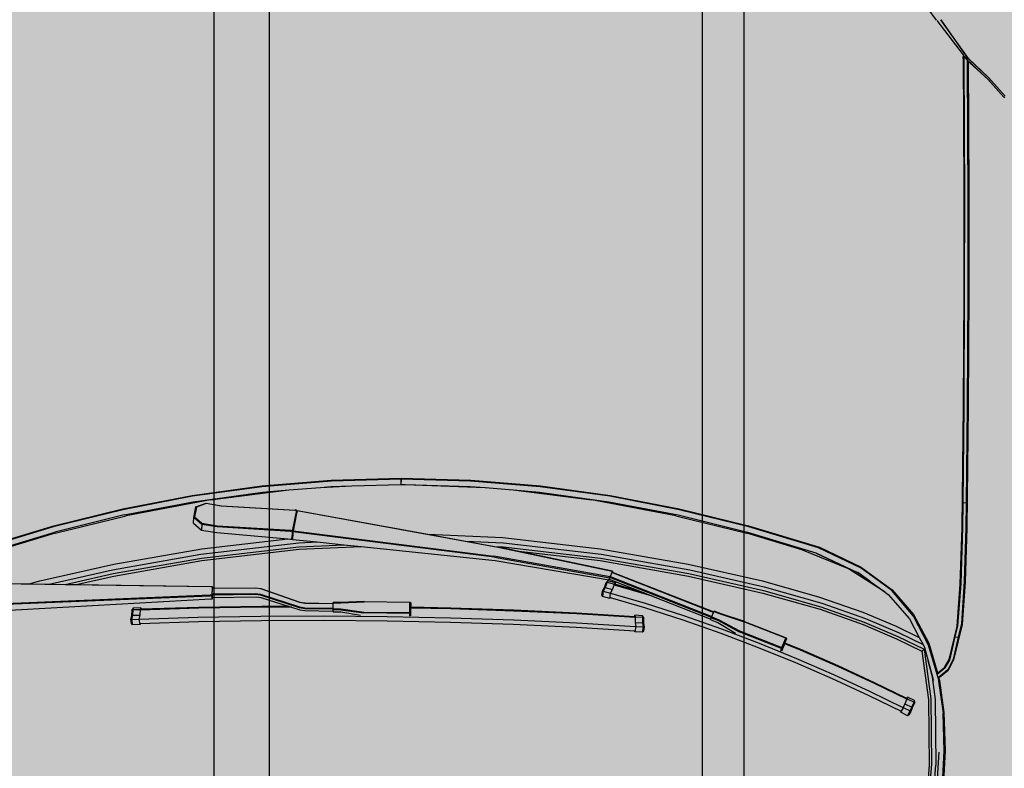
# Model space of a CAD drawing. Units: inches. Extents: x 1884 to 2398, y 474 to 1488.
# Tile 28 of 39: x 2306 to 2356, y 699 to 737. Entities that reach past the tile are written whole.
import ezdxf

# ---------------------------------------------------------------- set-up
doc = ezdxf.new("R2010")
doc.units = ezdxf.units.IN
doc.header["$MEASUREMENT"] = 0
doc.layers.get('0').update_dxf_attribs({"color": 250})
doc.layers.add('A-ANNO-DIMS', color=2, linetype='Continuous', lineweight=18)
doc.layers.add('C-VEHI', color=8, linetype='Continuous', lineweight=18)
doc.layers.add('Edges', color=250, linetype='Continuous')
doc.layers.add('L-PVMT-PATT', color=9, linetype='Continuous', lineweight=13, true_color=0xc7c8ca)
doc.styles.get("Standard").update_dxf_attribs({"font": 'arial.ttf'})
doc.dimstyles.get("Standard").update_dxf_attribs({"dimtxt": 7, "dimasz": 0.18, "dimexe": 0.18, "dimexo": 0.0625, "dimgap": 0.09, "dimtad": 0, "dimtih": 1, "dimtoh": 1, "dimzin": 0, "dimdsep": 46, "dimlunit": 3, "dimtxsty": 'Standard', "dimcen": 0.09, "dimadec": 0, "dimazin": 0, "dimtfac": 1, "dimtofl": 0, "dimtmove": 0, "dimatfit": 3, "dimfxl": 1, "dimtolj": 1, "dimtzin": 0, "dimarcsym": 0})

# ---------------------------------------------------------------- blocks, each defined once
blk = doc.blocks.new('Nissan Qashqai pl')
at = {"layer": 'Edges'}
for p, q in [((7.7748, 12.7018), (7.7507, 12.6803)), ((7.753, 12.6794), (7.776, 12.6999)), ((7.776, 12.6999), (7.7539, 12.68)), ((7.7772, 12.7011), (7.776, 12.6999)), ((7.7261, 12.6543), (7.7507, 12.6803)), ((7.7507, 12.6803), (7.7286, 12.6561)), ((7.7539, 12.68), (7.7324, 12.6565)), ((7.753, 12.6794), (7.7281, 12.6524)), ((7.7286, 12.6561), (7.7267, 12.6539)), ((7.7324, 12.6565), (7.7299, 12.6537)), ((7.8083, 12.6544), (7.904, 12.6547)), ((7.904, 12.6547), (8.0276, 12.6545)), ((8.0276, 12.6545), (8.1753, 12.6539)), ((7.7261, 12.6543), (7.6762, 12.6186)), ((7.6762, 12.6186), (7.7233, 12.6514)), ((7.6771, 12.6135), (7.7215, 12.6473)), ((7.7215, 12.6473), (7.7221, 12.6478)), ((7.7232, 12.6486), (7.7221, 12.6478)), ((7.7281, 12.6524), (7.7232, 12.6486)), ((7.7245, 12.6486), (7.7232, 12.6486)), ((7.7267, 12.6539), (7.7233, 12.6514)), ((7.7261, 12.6476), (7.7238, 12.6476)), ((7.7294, 12.6487), (7.7245, 12.6486)), ((7.7279, 12.6477), (7.7261, 12.6476)), ((7.8048, 12.6483), (7.7279, 12.6477)), ((7.7299, 12.6537), (7.7281, 12.6524)), ((7.7281, 12.6524), (7.7349, 12.6524)), ((7.731, 12.6487), (7.7294, 12.6487)), ((7.7299, 12.6537), (7.7334, 12.6537)), ((7.764, 12.6489), (7.731, 12.6487)), ((7.7334, 12.6537), (7.8083, 12.6544)), ((7.7349, 12.6524), (7.768, 12.6527)), ((7.7662, 12.6489), (7.764, 12.6489)), ((7.7811, 12.649), (7.7662, 12.6489)), ((7.768, 12.6527), (7.7692, 12.6527)), ((7.7692, 12.6527), (7.7844, 12.6528)), ((7.7822, 12.649), (7.7811, 12.649)), ((7.8057, 12.6491), (7.7822, 12.649)), ((7.7844, 12.6528), (7.8078, 12.653)), ((7.9014, 12.6487), (7.8048, 12.6483)), ((7.8233, 12.6492), (7.8057, 12.6491)), ((7.8078, 12.653), (7.8233, 12.6531)), ((7.8233, 12.6531), (7.9036, 12.6534)), ((7.902, 12.6495), (7.8233, 12.6492)), ((8.0273, 12.6485), (7.9014, 12.6487)), ((8.0275, 12.6493), (7.902, 12.6495)), ((7.9036, 12.6534), (8.0275, 12.6533)), ((8.1753, 12.6479), (8.0273, 12.6485)), ((8.0275, 12.6533), (8.1755, 12.6527)), ((8.1754, 12.6487), (8.0275, 12.6493)), ((8.1753, 12.6539), (8.3324, 12.6521)), ((8.3318, 12.6462), (8.1753, 12.6479)), ((8.3002, 12.6474), (8.1754, 12.6487)), ((8.1755, 12.6527), (8.3005, 12.6514)), ((8.3005, 12.6514), (8.3002, 12.6474)), ((8.332, 12.6471), (8.3002, 12.6474)), ((8.3005, 12.6514), (8.3324, 12.651)), ((8.4049, 12.6437), (8.3318, 12.6462)), ((8.4042, 12.6447), (8.332, 12.6471)), ((8.3324, 12.6521), (8.4022, 12.6498)), ((8.3324, 12.651), (8.4014, 12.6488)), ((8.4014, 12.6488), (8.4559, 12.6451)), ((8.4022, 12.6498), (8.4571, 12.6459)), ((8.4588, 12.6405), (8.4042, 12.6447)), ((8.4595, 12.6395), (8.4049, 12.6437)), ((8.4559, 12.6451), (8.4736, 12.6409)), ((8.4571, 12.6459), (8.5029, 12.635)), ((8.4729, 12.6372), (8.4588, 12.6405)), ((8.5025, 12.6293), (8.4595, 12.6395)), ((8.4729, 12.6372), (8.4736, 12.6409)), ((8.5032, 12.6301), (8.4729, 12.6372)), ((8.4736, 12.6409), (8.5018, 12.6344)), ((8.5018, 12.6344), (8.5155, 12.6274)), ((8.5125, 12.6231), (8.5025, 12.6293)), ((8.5029, 12.635), (8.5163, 12.6279)), ((8.5132, 12.624), (8.5032, 12.6301)), ((8.5177, 12.617), (8.5125, 12.6231)), ((8.5132, 12.624), (8.5216, 12.6139)), ((8.5155, 12.6274), (8.5258, 12.6151)), ((8.5163, 12.6279), (8.5237, 12.6189)), ((8.5197, 12.6145), (8.5177, 12.617)), ((8.5237, 12.6189), (8.5259, 12.6162)), ((8.5259, 12.6162), (8.5294, 12.6167)), ((8.5294, 12.6167), (8.5706, 12.6226)), ((8.5304, 12.6157), (8.5715, 12.6215)), ((8.5706, 12.6226), (8.6197, 12.6241)), ((8.6203, 12.6229), (8.5715, 12.6215)), ((8.6197, 12.6241), (8.6683, 12.6215)), ((8.6203, 12.6229), (8.6204, 12.6229)), ((8.6721, 12.6201), (8.6204, 12.6229)), ((7.6769, 12.6129), (7.6306, 12.5791)), ((8.4814, 12.6029), (8.5166, 12.6135)), ((8.5216, 12.6139), (8.4838, 12.6027)), ((8.4889, 12.5969), (8.5531, 12.6055)), ((8.5039, 12.6023), (8.528, 12.6088)), ((8.5216, 12.6068), (8.5039, 12.6023)), ((8.5166, 12.6135), (8.5197, 12.6145)), ((8.5197, 12.6145), (8.5216, 12.6139)), ((8.5258, 12.6151), (8.5216, 12.6139)), ((8.5216, 12.6068), (8.5538, 12.6111)), ((8.5301, 12.609), (8.5216, 12.6068)), ((8.5259, 12.6162), (8.5258, 12.6151)), ((8.5258, 12.6151), (8.5304, 12.6157)), ((8.5304, 12.6157), (8.5304, 12.6157)), ((8.5531, 12.6055), (8.6375, 12.6066)), ((8.5538, 12.6111), (8.6387, 12.6123)), ((8.5544, 12.6026), (8.6386, 12.6037)), ((8.622, 12.6161), (8.6699, 12.6132)), ((8.6375, 12.6066), (8.7481, 12.5968)), ((8.6386, 12.6037), (8.7491, 12.594)), ((8.6721, 12.6093), (8.6387, 12.6123)), ((8.4444, 12.5834), (8.4814, 12.6029)), ((8.4838, 12.6027), (8.4462, 12.5833)), ((8.468, 12.5648), (8.4831, 12.5957)), ((8.4725, 12.563), (8.4889, 12.5969)), ((8.4737, 12.5908), (8.4831, 12.5957)), ((8.4756, 12.5615), (8.4914, 12.5942)), ((8.4831, 12.5957), (8.4867, 12.5977)), ((8.4867, 12.5977), (8.5039, 12.6023)), ((8.4914, 12.5942), (8.4889, 12.5969)), ((8.4914, 12.5942), (8.5544, 12.6026)), ((8.4122, 12.5558), (8.4444, 12.5834)), ((8.4462, 12.5833), (8.4134, 12.5554)), ((8.4499, 12.5782), (8.4737, 12.5908)), ((8.4594, 12.5611), (8.4737, 12.5908)), ((8.5554, 12.5847), (8.551, 12.5757)), ((8.5529, 12.5751), (8.5572, 12.5841)), ((8.5574, 12.5849), (8.5554, 12.5847)), ((8.5572, 12.5841), (8.5554, 12.5847)), ((8.5639, 12.581), (8.5572, 12.5841)), ((8.5574, 12.5849), (8.5584, 12.5846)), ((8.5582, 12.5845), (8.5574, 12.5849)), ((8.5584, 12.5846), (8.5649, 12.5816)), ((8.5595, 12.572), (8.5639, 12.581)), ((8.5687, 12.5791), (8.5639, 12.581)), ((8.5644, 12.5701), (8.5687, 12.5791)), ((8.5649, 12.5816), (8.5693, 12.5799)), ((8.5687, 12.5791), (8.5693, 12.5799)), ((8.5749, 12.5757), (8.5687, 12.5791)), ((8.5693, 12.5799), (8.5739, 12.5774)), ((8.4183, 12.5508), (8.4499, 12.5782)), ((8.5527, 12.5749), (8.5323, 12.5332)), ((8.5537, 12.5747), (8.5332, 12.5329)), ((8.5647, 12.57), (8.5441, 12.5279)), ((8.5487, 12.5256), (8.5692, 12.5674)), ((8.5527, 12.5749), (8.551, 12.5757)), ((8.551, 12.5757), (8.5528, 12.5751)), ((8.5528, 12.5751), (8.5527, 12.5749)), ((8.5528, 12.5751), (8.5529, 12.5751)), ((8.5529, 12.5751), (8.5537, 12.5747)), ((8.5537, 12.5747), (8.5595, 12.572)), ((8.5595, 12.572), (8.5644, 12.5701)), ((8.5644, 12.5701), (8.5647, 12.57)), ((8.5647, 12.57), (8.5692, 12.5675)), ((8.5692, 12.5674), (8.5692, 12.5675)), ((8.5692, 12.5675), (8.5705, 12.5668)), ((8.5705, 12.5668), (8.5692, 12.5674)), ((8.5749, 12.5757), (8.5705, 12.5668)), ((8.5739, 12.5774), (8.5749, 12.5757)), ((8.3826, 12.5151), (8.4122, 12.5558)), ((8.4134, 12.5554), (8.3844, 12.5157)), ((8.4411, 12.5178), (8.4594, 12.5611)), ((8.4493, 12.5212), (8.468, 12.5648)), ((8.454, 12.5196), (8.4725, 12.563)), ((8.4571, 12.5184), (8.4756, 12.5615)), ((8.4154, 12.5468), (8.3852, 12.4994)), ((8.3901, 12.5113), (8.4154, 12.5468)), ((8.4011, 12.5269), (8.4154, 12.5468)), ((8.4156, 12.547), (8.4154, 12.5468)), ((8.4156, 12.547), (8.4183, 12.5508)), ((8.5323, 12.5332), (8.5103, 12.4859)), ((8.5332, 12.5329), (8.5112, 12.4856)), ((8.5441, 12.5279), (8.5222, 12.4807)), ((8.3573, 12.4618), (8.3826, 12.5151)), ((8.3844, 12.5157), (8.3582, 12.4606)), ((8.4011, 12.5269), (8.3901, 12.5113)), ((8.3904, 12.512), (8.4011, 12.5269)), ((8.4217, 12.4622), (8.4411, 12.5178)), ((8.4296, 12.4651), (8.4493, 12.5212)), ((8.4343, 12.4637), (8.454, 12.5196)), ((8.4375, 12.4627), (8.4571, 12.5184)), ((8.5269, 12.4785), (8.5487, 12.5256)), ((8.3646, 12.4572), (8.39, 12.5111)), ((8.3648, 12.4579), (8.39, 12.5111)), ((8.39, 12.5111), (8.3852, 12.4994)), ((8.39, 12.5111), (8.3901, 12.5113)), ((8.3901, 12.5113), (8.3904, 12.512)), ((8.3852, 12.4994), (8.3608, 12.4393)), ((8.5103, 12.4859), (8.4895, 12.4381)), ((8.5112, 12.4856), (8.4904, 12.4377)), ((8.5222, 12.4807), (8.5014, 12.4329)), ((8.5062, 12.431), (8.5269, 12.4785)), ((8.4084, 12.3907), (8.4296, 12.4651)), ((8.3296, 12.3703), (8.3573, 12.4618)), ((8.3582, 12.4606), (8.3311, 12.3708)), ((8.3377, 12.3689), (8.3646, 12.4572)), ((8.3646, 12.4572), (8.3648, 12.4579)), ((8.3648, 12.4579), (8.3648, 12.4579)), ((8.4009, 12.3883), (8.4217, 12.4622)), ((8.4133, 12.3896), (8.4343, 12.4637)), ((8.4165, 12.3888), (8.4375, 12.4627)), ((8.3608, 12.4393), (8.3392, 12.3684)), ((8.3608, 12.4393), (8.3608, 12.4393)), ((8.4895, 12.4381), (8.4811, 12.4174)), ((8.5014, 12.4329), (8.4817, 12.3847)), ((8.4904, 12.4377), (8.482, 12.4171)), ((8.4866, 12.3829), (8.5062, 12.431)), ((8.4526, 12.3639), (8.4742, 12.4188)), ((8.4747, 12.4185), (8.4532, 12.3636)), ((8.4654, 12.3587), (8.4869, 12.4136)), ((8.4742, 12.4188), (8.4754, 12.4193)), ((8.4747, 12.4185), (8.4742, 12.4188)), ((8.4754, 12.4193), (8.4747, 12.4185)), ((8.4869, 12.4136), (8.4747, 12.4185)), ((8.4754, 12.4193), (8.4876, 12.4144)), ((8.4791, 12.4183), (8.4754, 12.4193)), ((8.4811, 12.4174), (8.4791, 12.4183)), ((8.482, 12.4171), (8.4811, 12.4174)), ((8.4912, 12.4133), (8.482, 12.4171)), ((8.4869, 12.4136), (8.4876, 12.4144)), ((8.4881, 12.4131), (8.4869, 12.4136)), ((8.4876, 12.4144), (8.4912, 12.4133)), ((8.4876, 12.4144), (8.4881, 12.4131)), ((8.4913, 12.4133), (8.4912, 12.4133)), ((8.4913, 12.4132), (8.4913, 12.4133)), ((8.4881, 12.4131), (8.4666, 12.3582)), ((8.4914, 12.4121), (8.4881, 12.4131)), ((8.3792, 12.2926), (8.4009, 12.3883)), ((8.3864, 12.2945), (8.4084, 12.3907)), ((8.3913, 12.2935), (8.4133, 12.3896)), ((8.3945, 12.2929), (8.4165, 12.3888)), ((8.4817, 12.3847), (8.4633, 12.3359)), ((8.4683, 12.3345), (8.4866, 12.3829)), ((8.3076, 12.281), (8.3296, 12.3703)), ((8.3311, 12.3708), (8.3089, 12.2811)), ((8.3157, 12.2795), (8.3377, 12.3689)), ((8.3166, 12.2767), (8.3392, 12.3684)), ((8.4526, 12.3639), (8.4434, 12.3353)), ((8.4439, 12.335), (8.4532, 12.3636)), ((8.4509, 12.3322), (8.4654, 12.3587)), ((8.4521, 12.3317), (8.4666, 12.3582)), ((8.4547, 12.3309), (8.4682, 12.3538)), ((8.3894, 12.1944), (8.4409, 12.3255)), ((8.4415, 12.3252), (8.3899, 12.1941)), ((8.4434, 12.3353), (8.4397, 12.326)), ((8.4403, 12.3257), (8.4397, 12.326)), ((8.4403, 12.3257), (8.4439, 12.335)), ((8.4409, 12.3255), (8.4403, 12.3257)), ((8.4415, 12.3252), (8.4409, 12.3255)), ((8.4467, 12.3231), (8.4415, 12.3252)), ((8.4633, 12.3359), (8.4461, 12.2868)), ((8.4472, 12.3229), (8.4509, 12.3322)), ((8.4484, 12.3224), (8.4521, 12.3317)), ((8.4511, 12.3216), (8.4547, 12.3309)), ((8.4512, 12.2856), (8.4683, 12.3345)), ((8.3951, 12.192), (8.4467, 12.3231)), ((8.4479, 12.3226), (8.3963, 12.1915)), ((8.4209, 12.2475), (8.4502, 12.3219)), ((8.4472, 12.3229), (8.4467, 12.3231)), ((8.4479, 12.3226), (8.4472, 12.3229)), ((8.4484, 12.3224), (8.4479, 12.3226)), ((8.4502, 12.3219), (8.4484, 12.3224)), ((8.4511, 12.3216), (8.4502, 12.3219)), ((8.3593, 12.1791), (8.3792, 12.2926)), ((8.3662, 12.1803), (8.3864, 12.2945)), ((8.3713, 12.1796), (8.3913, 12.2935)), ((8.3745, 12.1792), (8.3945, 12.2929)), ((8.4461, 12.2868), (8.4302, 12.2373)), ((8.2905, 12.1918), (8.3076, 12.281)), ((8.3089, 12.2811), (8.2916, 12.1913)), ((8.3166, 12.2767), (8.296, 12.168)), ((8.2985, 12.1901), (8.3157, 12.2795)), ((8.4353, 12.2363), (8.4512, 12.2856)), ((8.3986, 12.1908), (8.4163, 12.2359)), ((8.4163, 12.2359), (8.4052, 12.1979)), ((8.4191, 12.2418), (8.4061, 12.1973)), ((8.4163, 12.2359), (8.4209, 12.2475)), ((8.4302, 12.2373), (8.4171, 12.1926)), ((8.4209, 12.2475), (8.4191, 12.2418)), ((8.4224, 12.1919), (8.4353, 12.2363)), ((8.4557, 12.235), (8.4603, 12.2357)), ((8.46, 12.2348), (8.4603, 12.2357)), ((8.4603, 12.2357), (8.4655, 12.2348)), ((8.4471, 12.2238), (8.4425, 12.1485)), ((8.448, 12.2241), (8.4435, 12.1487)), ((8.4457, 12.2337), (8.4452, 12.2238)), ((8.4452, 12.2238), (8.4471, 12.2242)), ((8.4471, 12.2238), (8.4452, 12.2238)), ((8.4475, 12.2348), (8.4457, 12.2337)), ((8.4476, 12.2341), (8.4457, 12.2337)), ((8.4471, 12.2242), (8.4476, 12.2341)), ((8.4471, 12.2242), (8.4544, 12.2242)), ((8.4471, 12.2239), (8.4471, 12.2238)), ((8.4475, 12.2348), (8.4484, 12.235)), ((8.4555, 12.2348), (8.4475, 12.2348)), ((8.4549, 12.2341), (8.4476, 12.2341)), ((8.4484, 12.235), (8.4557, 12.235)), ((8.4544, 12.2242), (8.4549, 12.2341)), ((8.4544, 12.2242), (8.4595, 12.2249)), ((8.46, 12.2348), (8.4549, 12.2341)), ((8.4601, 12.2247), (8.4555, 12.1488)), ((8.4595, 12.2249), (8.46, 12.2348)), ((8.4595, 12.2249), (8.4666, 12.2237)), ((8.4671, 12.2337), (8.46, 12.2348)), ((8.4607, 12.1481), (8.4652, 12.2237)), ((8.4652, 12.2237), (8.4652, 12.2238)), ((8.4666, 12.2237), (8.4652, 12.2237)), ((8.4655, 12.2348), (8.4671, 12.2337)), ((8.4671, 12.2337), (8.4666, 12.2237)), ((8.4035, 12.1986), (8.4007, 12.189)), ((8.4023, 12.1879), (8.4052, 12.1975)), ((8.4052, 12.1975), (8.4035, 12.1986)), ((8.4035, 12.1986), (8.4052, 12.1979)), ((8.4052, 12.1979), (8.4052, 12.1978)), ((8.412, 12.195), (8.4052, 12.1975)), ((8.2781, 12.1018), (8.2905, 12.1918)), ((8.2916, 12.1913), (8.2793, 12.1016)), ((8.2862, 12.1008), (8.2985, 12.1901)), ((8.3887, 12.1946), (8.3575, 12.0475)), ((8.3882, 12.1948), (8.3618, 12.07)), ((8.3957, 12.1917), (8.3688, 12.0419)), ((8.3702, 12.0427), (8.3969, 12.1913)), ((8.3746, 12.0435), (8.3995, 12.1905)), ((8.3887, 12.1946), (8.3882, 12.1948)), ((8.3882, 12.1948), (8.3894, 12.1944)), ((8.3894, 12.1944), (8.3887, 12.1946)), ((8.3894, 12.1944), (8.3894, 12.1944)), ((8.3894, 12.1944), (8.3899, 12.1941)), ((8.3899, 12.1941), (8.3951, 12.192)), ((8.3951, 12.192), (8.3963, 12.1915)), ((8.3957, 12.1917), (8.3951, 12.192)), ((8.3969, 12.1913), (8.3957, 12.1917)), ((8.3963, 12.1915), (8.3986, 12.1908)), ((8.3995, 12.1905), (8.3969, 12.1913)), ((8.3995, 12.1905), (8.3986, 12.1908)), ((8.4007, 12.189), (8.4023, 12.1879)), ((8.4007, 12.189), (8.402, 12.1874)), ((8.4028, 12.1868), (8.402, 12.1874)), ((8.402, 12.1874), (8.4027, 12.1871)), ((8.4023, 12.1879), (8.4092, 12.1855)), ((8.4097, 12.1844), (8.4028, 12.1868)), ((8.4092, 12.1855), (8.412, 12.195)), ((8.4092, 12.1855), (8.4139, 12.1829)), ((8.4167, 12.1925), (8.412, 12.195)), ((8.4139, 12.1829), (8.4167, 12.1925)), ((8.4237, 12.1914), (8.4167, 12.1925)), ((8.4237, 12.1914), (8.4209, 12.1819)), ((8.4223, 12.1918), (8.4224, 12.1919)), ((8.4224, 12.1919), (8.4237, 12.1914)), ((8.3448, 12.0536), (8.3593, 12.1791)), ((8.3516, 12.0542), (8.3662, 12.1803)), ((8.3567, 12.0538), (8.3713, 12.1796)), ((8.3618, 12.07), (8.3745, 12.1792)), ((8.4139, 12.1821), (8.4097, 12.1844)), ((8.4139, 12.1829), (8.4209, 12.1819)), ((8.4139, 12.1821), (8.4139, 12.1829)), ((8.4191, 12.1813), (8.4139, 12.1821)), ((8.4209, 12.1819), (8.4191, 12.1813)), ((8.2834, 12.0669), (8.296, 12.168)), ((8.4425, 12.1485), (8.4387, 12.0674)), ((8.4435, 12.1487), (8.4397, 12.0674)), ((8.4555, 12.1488), (8.4517, 12.0674)), ((8.4568, 12.0669), (8.4607, 12.1481)), ((8.2708, 12.0123), (8.2781, 12.1018)), ((8.2793, 12.1016), (8.2719, 12.0118)), ((8.2834, 12.0669), (8.2862, 12.1008)), ((8.2804, 12.0305), (8.2834, 12.0669)), ((8.3618, 12.07), (8.3574, 12.0489)), ((8.4387, 12.0674), (8.4359, 11.9861)), ((8.4397, 12.0674), (8.4369, 11.9861)), ((8.4517, 12.0674), (8.4489, 11.9858)), ((8.4541, 11.9857), (8.4568, 12.0669)), ((8.3575, 12.0475), (8.3104, 11.7881)), ((8.3406, 11.9567), (8.3448, 12.0536)), ((8.3495, 12.0053), (8.3516, 12.0542)), ((8.3562, 12.0421), (8.3567, 12.0538)), ((8.3562, 12.0421), (8.3574, 12.0489)), ((8.336, 11.7828), (8.3688, 12.0419)), ((8.3702, 12.0427), (8.3374, 11.7826)), ((8.3495, 12.0053), (8.3562, 12.0421)), ((8.3565, 11.8707), (8.3746, 12.0435)), ((8.2765, 11.9273), (8.2804, 12.0305)), ((8.2788, 12.0114), (8.2804, 12.0305)), ((8.2682, 11.9221), (8.2708, 12.0123)), ((8.2719, 12.0118), (8.2695, 11.9221)), ((8.2765, 11.9273), (8.2788, 12.0114)), ((8.3406, 11.9567), (8.3495, 12.0053)), ((8.4359, 11.9861), (8.4348, 11.9346)), ((8.4369, 11.9861), (8.4358, 11.9346)), ((8.4489, 11.9858), (8.4471, 11.9043)), ((8.4523, 11.9043), (8.4541, 11.9857)), ((8.31, 11.7882), (8.3406, 11.9567)), ((8.4272, 11.8746), (8.4281, 11.9336)), ((8.4287, 11.9335), (8.4278, 11.8745)), ((8.4281, 11.9336), (8.429, 11.9345)), ((8.4281, 11.9336), (8.4287, 11.9336)), ((8.4287, 11.9335), (8.4281, 11.9336)), ((8.429, 11.9345), (8.4287, 11.9336)), ((8.4287, 11.9336), (8.4287, 11.9335)), ((8.4418, 11.9332), (8.4287, 11.9335)), ((8.4328, 11.9347), (8.429, 11.9345)), ((8.429, 11.9345), (8.4326, 11.9345)), ((8.4328, 11.9347), (8.4326, 11.9345)), ((8.4326, 11.9345), (8.4348, 11.9344)), ((8.4348, 11.9346), (8.4328, 11.9347)), ((8.4348, 11.9346), (8.4348, 11.9344)), ((8.4358, 11.9346), (8.4348, 11.9346)), ((8.4348, 11.9344), (8.4358, 11.9344)), ((8.4358, 11.9346), (8.4358, 11.9344)), ((8.4459, 11.9344), (8.4358, 11.9346)), ((8.4358, 11.9344), (8.4422, 11.9342)), ((8.441, 11.8742), (8.4418, 11.9332)), ((8.4418, 11.9332), (8.4422, 11.9342)), ((8.4431, 11.9332), (8.4418, 11.9332)), ((8.4422, 11.9342), (8.4459, 11.9344)), ((8.4422, 11.9342), (8.4431, 11.9332)), ((8.4431, 11.9332), (8.4422, 11.8742)), ((8.4464, 11.9334), (8.4431, 11.9332)), ((8.4459, 11.9344), (8.4459, 11.9344)), ((8.2708, 11.8319), (8.2682, 11.9221)), ((8.2763, 11.9223), (8.2695, 11.9221)), ((8.2695, 11.9221), (8.2763, 11.9219)), ((8.2695, 11.9221), (8.2719, 11.8323)), ((8.2763, 11.9223), (8.2764, 11.9263)), ((8.2763, 11.9219), (8.2763, 11.9223)), ((8.2781, 11.8585), (8.2763, 11.9219)), ((8.2764, 11.9263), (8.2765, 11.9273)), ((8.4471, 11.9043), (8.4464, 11.8227)), ((8.4516, 11.823), (8.4523, 11.9043)), ((8.3542, 11.8485), (8.3565, 11.8707)), ((8.3599, 11.7906), (8.3565, 11.8707)), ((8.4272, 11.8746), (8.4286, 11.8445)), ((8.4292, 11.8445), (8.4278, 11.8745)), ((8.4368, 11.8443), (8.441, 11.8742)), ((8.438, 11.8443), (8.4422, 11.8742)), ((8.4408, 11.8444), (8.4452, 11.8698)), ((8.28, 11.818), (8.2781, 11.8585)), ((8.2788, 11.8327), (8.2781, 11.8585)), ((8.2789, 11.8319), (8.2781, 11.8585)), ((8.3505, 11.8139), (8.3542, 11.8485)), ((8.3567, 11.7903), (8.3542, 11.8485)), ((8.4286, 11.8445), (8.4285, 11.8345)), ((8.4291, 11.8345), (8.4292, 11.8445)), ((8.4366, 11.8345), (8.4368, 11.8443)), ((8.4379, 11.8345), (8.438, 11.8443)), ((8.4406, 11.8344), (8.4408, 11.8444)), ((8.2781, 11.7423), (8.2708, 11.8319)), ((8.2719, 11.8323), (8.2793, 11.7426)), ((8.2789, 11.8319), (8.2788, 11.8327)), ((8.28, 11.818), (8.2789, 11.8319)), ((8.4291, 11.8345), (8.4285, 11.8345)), ((8.4298, 11.8345), (8.4291, 11.8345)), ((8.4292, 11.7978), (8.4298, 11.8345)), ((8.4304, 11.8345), (8.4298, 11.7978)), ((8.4304, 11.8345), (8.4298, 11.8345)), ((8.436, 11.8344), (8.4304, 11.8345)), ((8.4355, 11.7977), (8.436, 11.8344)), ((8.4366, 11.8343), (8.436, 11.8344)), ((8.4366, 11.8345), (8.4379, 11.8345)), ((8.4366, 11.8344), (8.4366, 11.8345)), ((8.4373, 11.8344), (8.4366, 11.8344)), ((8.4373, 11.8344), (8.4366, 11.8343)), ((8.4366, 11.8343), (8.4366, 11.8344)), ((8.4373, 11.8344), (8.4367, 11.7977)), ((8.4379, 11.8344), (8.4373, 11.8344)), ((8.4379, 11.8343), (8.4373, 11.8344)), ((8.4379, 11.8344), (8.4379, 11.8345)), ((8.4397, 11.8344), (8.4379, 11.8343)), ((8.4379, 11.8343), (8.4379, 11.8344)), ((8.4391, 11.7978), (8.4397, 11.8344)), ((8.4406, 11.8344), (8.4397, 11.8344)), ((8.2834, 11.7773), (8.28, 11.818)), ((8.4464, 11.8227), (8.4468, 11.7413)), ((8.452, 11.7418), (8.4516, 11.823)), ((8.3472, 11.7821), (8.3505, 11.8139)), ((8.3516, 11.79), (8.3505, 11.8139)), ((8.3745, 11.665), (8.3599, 11.7906)), ((8.4107, 11.7411), (8.4281, 11.7914)), ((8.4287, 11.7914), (8.4111, 11.741)), ((8.4179, 11.7406), (8.4344, 11.7912)), ((8.4357, 11.7912), (8.4193, 11.7407)), ((8.4281, 11.7914), (8.4292, 11.7978)), ((8.4298, 11.7978), (8.4287, 11.7914)), ((8.4344, 11.7912), (8.4355, 11.7977)), ((8.4347, 11.7805), (8.4381, 11.7914)), ((8.4367, 11.7977), (8.4357, 11.7912)), ((8.4381, 11.7914), (8.4391, 11.7978)), ((8.3038, 11.6903), (8.3095, 11.7853)), ((8.3099, 11.7851), (8.3042, 11.6901)), ((8.3092, 11.7863), (8.3093, 11.7873)), ((8.3092, 11.7863), (8.3099, 11.7851)), ((8.3095, 11.7853), (8.3092, 11.7863)), ((8.3093, 11.7873), (8.3367, 11.7816)), ((8.3159, 11.7869), (8.3093, 11.7873)), ((8.31, 11.7882), (8.3104, 11.7881)), ((8.3104, 11.7881), (8.3159, 11.7869)), ((8.3159, 11.7869), (8.336, 11.7828)), ((8.3298, 11.6848), (8.3355, 11.7798)), ((8.3369, 11.7796), (8.3312, 11.6846)), ((8.3355, 11.7798), (8.3366, 11.7806)), ((8.336, 11.7828), (8.3374, 11.7826)), ((8.3367, 11.7816), (8.3366, 11.7806)), ((8.3366, 11.7806), (8.3369, 11.7796)), ((8.3367, 11.7816), (8.347, 11.7811)), ((8.3374, 11.7826), (8.3406, 11.7824)), ((8.3458, 11.7813), (8.3406, 11.7824)), ((8.3406, 11.7824), (8.3457, 11.7821)), ((8.3458, 11.7813), (8.3457, 11.7821)), ((8.3457, 11.7821), (8.3472, 11.7821)), ((8.347, 11.7811), (8.3458, 11.7813)), ((8.3464, 11.7761), (8.3467, 11.7791)), ((8.3467, 11.7791), (8.347, 11.7811)), ((8.3662, 11.6639), (8.3516, 11.79)), ((8.3713, 11.6645), (8.3567, 11.7903)), ((8.4337, 11.7775), (8.4347, 11.7805)), ((8.4347, 11.7805), (8.4348, 11.7421)), ((8.296, 11.6762), (8.2834, 11.7773)), ((8.2862, 11.7434), (8.2834, 11.7773)), ((8.3385, 11.6842), (8.3464, 11.7761)), ((8.3593, 11.6651), (8.3464, 11.7761)), ((8.4222, 11.7413), (8.4337, 11.7775)), ((8.4337, 11.7775), (8.4339, 11.7423)), ((8.2905, 11.6524), (8.2781, 11.7423)), ((8.2793, 11.7426), (8.2916, 11.6528)), ((8.2985, 11.654), (8.2862, 11.7434)), ((8.4097, 11.7348), (8.4107, 11.7411)), ((8.4111, 11.741), (8.41, 11.7346)), ((8.417, 11.7342), (8.4179, 11.7406)), ((8.4193, 11.7407), (8.4183, 11.7343)), ((8.4213, 11.735), (8.4222, 11.7413)), ((8.4339, 11.7423), (8.4353, 11.6613)), ((8.4348, 11.7421), (8.4362, 11.661)), ((8.4468, 11.7413), (8.4482, 11.66)), ((8.4534, 11.6608), (8.452, 11.7418)), ((8.4104, 11.6791), (8.4097, 11.7348)), ((8.41, 11.7346), (8.4108, 11.6791)), ((8.4177, 11.678), (8.417, 11.7342)), ((8.4183, 11.7343), (8.4191, 11.678)), ((8.4221, 11.6787), (8.4213, 11.735)), ((8.3005, 11.6706), (8.3038, 11.6903)), ((8.3042, 11.6901), (8.3009, 11.6704)), ((8.3264, 11.6652), (8.3298, 11.6848)), ((8.3312, 11.6846), (8.3278, 11.665)), ((8.3352, 11.6646), (8.3385, 11.6842)), ((8.4086, 11.6764), (8.4045, 11.4011)), ((8.4056, 11.5028), (8.4082, 11.6766)), ((8.4082, 11.6785), (8.4104, 11.6791)), ((8.4082, 11.6785), (8.4086, 11.6784)), ((8.4082, 11.6766), (8.4082, 11.6785)), ((8.4086, 11.6784), (8.4086, 11.6764)), ((8.4086, 11.6784), (8.4117, 11.6782)), ((8.4104, 11.6791), (8.4108, 11.6791)), ((8.4104, 11.6786), (8.4104, 11.6791)), ((8.4108, 11.6786), (8.4104, 11.6786)), ((8.4104, 11.6786), (8.4108, 11.6784)), ((8.4108, 11.6791), (8.4108, 11.6786)), ((8.4108, 11.6786), (8.4108, 11.6784)), ((8.4108, 11.6784), (8.4117, 11.6783)), ((8.4117, 11.6783), (8.4117, 11.6782)), ((8.4117, 11.6783), (8.4177, 11.678)), ((8.4117, 11.6782), (8.419, 11.6778)), ((8.4177, 11.678), (8.4191, 11.678)), ((8.419, 11.6778), (8.4203, 11.6778)), ((8.419, 11.6758), (8.419, 11.6778)), ((8.4191, 11.678), (8.4221, 11.6787)), ((8.4238, 11.6786), (8.4203, 11.6778)), ((8.4203, 11.6778), (8.4204, 11.6758)), ((8.4238, 11.6786), (8.4221, 11.6787)), ((8.4238, 11.6766), (8.4238, 11.6786)), ((8.4394, 11.4014), (8.4238, 11.6766)), ((8.296, 11.6762), (8.3166, 11.5675)), ((8.3053, 11.6574), (8.3005, 11.6706)), ((8.3009, 11.6704), (8.3054, 11.6583)), ((8.3182, 11.6557), (8.3264, 11.6652)), ((8.3278, 11.665), (8.319, 11.6546)), ((8.3264, 11.6542), (8.3352, 11.6646)), ((8.3278, 11.665), (8.3352, 11.6646)), ((8.3792, 11.5515), (8.3593, 11.6651)), ((8.3864, 11.5497), (8.3662, 11.6639)), ((8.3913, 11.5506), (8.3713, 11.6645)), ((8.3945, 11.5513), (8.3745, 11.665)), ((8.4305, 11.3996), (8.419, 11.6758)), ((8.4204, 11.6758), (8.4319, 11.3996)), ((8.3076, 11.5631), (8.2905, 11.6524)), ((8.2916, 11.6528), (8.3089, 11.5631)), ((8.3157, 11.5647), (8.2985, 11.654)), ((8.3054, 11.6583), (8.3053, 11.6574)), ((8.319, 11.6546), (8.3053, 11.6574)), ((8.3054, 11.6583), (8.3182, 11.6557)), ((8.319, 11.6546), (8.3182, 11.6557)), ((8.3264, 11.6542), (8.319, 11.6546)), ((8.4353, 11.6613), (8.4375, 11.5863)), ((8.4362, 11.661), (8.4385, 11.5858)), ((8.4482, 11.66), (8.4505, 11.5843)), ((8.4557, 11.5855), (8.4534, 11.6608)), ((8.4377, 11.5857), (8.4357, 11.5864)), ((8.4357, 11.5864), (8.4359, 11.5765)), ((8.4357, 11.5864), (8.4375, 11.5863)), ((8.4359, 11.5765), (8.4379, 11.5758)), ((8.4359, 11.5765), (8.4377, 11.5753)), ((8.4375, 11.5863), (8.4375, 11.5862)), ((8.4379, 11.5758), (8.4377, 11.5857)), ((8.445, 11.5853), (8.4377, 11.5857)), ((8.4387, 11.5749), (8.4377, 11.5753)), ((8.4379, 11.5758), (8.4452, 11.5754)), ((8.4384, 11.5752), (8.4457, 11.5749)), ((8.446, 11.5746), (8.4387, 11.5749)), ((8.4452, 11.5754), (8.445, 11.5853)), ((8.4503, 11.5841), (8.445, 11.5853)), ((8.4452, 11.5754), (8.4505, 11.5742)), ((8.4507, 11.5734), (8.446, 11.5746)), ((8.4572, 11.5854), (8.4503, 11.5841)), ((8.4505, 11.5742), (8.4503, 11.5841)), ((8.4505, 11.5742), (8.4574, 11.5755)), ((8.4557, 11.5855), (8.4572, 11.5854)), ((8.4557, 11.5853), (8.4557, 11.5855)), ((8.4574, 11.5755), (8.4559, 11.5744)), ((8.4572, 11.5854), (8.4574, 11.5755)), ((8.3296, 11.4739), (8.3076, 11.5631)), ((8.3089, 11.5631), (8.3311, 11.4733)), ((8.3157, 11.5647), (8.3377, 11.4753)), ((8.3392, 11.4758), (8.3166, 11.5675)), ((8.4507, 11.5734), (8.4505, 11.5742)), ((8.4559, 11.5744), (8.4507, 11.5734)), ((8.4009, 11.4559), (8.3792, 11.5515)), ((8.4051, 11.4678), (8.3864, 11.5497)), ((8.4054, 11.4887), (8.3913, 11.5506)), ((8.4056, 11.5028), (8.3945, 11.5513)), ((8.4054, 11.4887), (8.4056, 11.5028)), ((8.4051, 11.4678), (8.4054, 11.4887)), ((8.3573, 11.3824), (8.3296, 11.4739)), ((8.3311, 11.4733), (8.3582, 11.3836)), ((8.3648, 11.3863), (8.3377, 11.4753)), ((8.3392, 11.4758), (8.3608, 11.4048)), ((8.4048, 11.4423), (8.4051, 11.4678)), ((8.4048, 11.4423), (8.4009, 11.4559)), ((8.4041, 11.4013), (8.4048, 11.4423))]:
    blk.add_line(p, q, dxfattribs=at)
blk = doc.blocks.new('car')
blk.add_blockref('Nissan Qashqai pl', (-9.7433, -11.9151))
blk = doc.blocks.new('carr')
blk.add_blockref('car', (0.5124, -0.007))
blk = doc.blocks.new('*D23')
at = {"layer": 'A-ANNO-DIMS', "color": 0, "lineweight": -2, "transparency": 16777216}
for p, q in [((2272.304, 752.812), (2298.291, 752.812)), ((2298.111, 752.632), (2298.111, 670.29)), ((2298.111, 580.529), (2298.111, 662.871)), ((2272.304, 580.349), (2298.291, 580.349))]:
    blk.add_line(p, q, dxfattribs=at)
at = {"layer": 'A-ANNO-DIMS', "color": 0, "lineweight": 100, "transparency": 16777216}
for points in [[(2298.081, 752.632), (2298.141, 752.632), (2298.111, 752.812)], [(2298.081, 580.529), (2298.141, 580.529), (2298.111, 580.349)]]:
    blk.add_solid(points, dxfattribs=at)
at = {"layer": 'Defpoints', "color": 0, "lineweight": 100, "transparency": 16777216}
for p in [(2272.242, 752.812), (2272.242, 580.349), (2298.111, 580.349)]:
    blk.add_point(p, dxfattribs=at)
at = {"layer": 'A-ANNO-DIMS', "color": 0, "transparency": 16777216, "insert": (2298.111, 666.58), "char_height": 7, "attachment_point": 5}
blk.add_mtext('\\A1;CAR 14\'-4 1/2" TYP.', dxfattribs=at)
blk = doc.blocks.new('*D47')
at = {"layer": 'A-ANNO-DIMS', "color": 0, "lineweight": -2, "transparency": 16777216}
for p, q in [((2315.591, 959.704), (2315.591, 484.005)), ((2342.529, 959.704), (2342.529, 484.005)), ((2315.771, 484.185), (2319.606, 484.185)), ((2342.349, 484.185), (2338.513, 484.185))]:
    blk.add_line(p, q, dxfattribs=at)
at = {"layer": 'A-ANNO-DIMS', "color": 0, "lineweight": 100, "transparency": 16777216}
for points in [[(2315.771, 484.215), (2315.771, 484.155), (2315.591, 484.185)], [(2342.349, 484.215), (2342.349, 484.155), (2342.529, 484.185)]]:
    blk.add_solid(points, dxfattribs=at)
at = {"layer": 'Defpoints', "color": 0, "lineweight": 100, "transparency": 16777216}
for p in [(2315.591, 959.766), (2342.529, 959.766), (2342.529, 484.185)]:
    blk.add_point(p, dxfattribs=at)
at = {"layer": 'A-ANNO-DIMS', "color": 0, "transparency": 16777216, "insert": (2329.06, 484.185), "char_height": 7, "attachment_point": 5}
blk.add_mtext('\\A1;2\'-3"', dxfattribs=at)
blk = doc.blocks.new('*D49')
at = {"layer": 'A-ANNO-DIMS', "color": 0, "lineweight": -2, "transparency": 16777216}
for p, q in [((2318.409, 987.716), (2318.409, 484.005)), ((2340.409, 987.716), (2340.409, 484.005)), ((2318.589, 484.185), (2340.229, 484.185)), ((2340.409, 484.185), (2340.589, 484.185))]:
    blk.add_line(p, q, dxfattribs=at)
at = {"layer": 'A-ANNO-DIMS', "color": 0, "lineweight": 100, "transparency": 16777216}
for points in [[(2318.589, 484.215), (2318.589, 484.155), (2318.409, 484.185)], [(2340.229, 484.215), (2340.229, 484.155), (2340.409, 484.185)]]:
    blk.add_solid(points, dxfattribs=at)
at = {"layer": 'Defpoints', "color": 0, "lineweight": 100, "transparency": 16777216}
for p in [(2318.409, 987.778), (2340.409, 987.778), (2340.409, 484.185)]:
    blk.add_point(p, dxfattribs=at)
at = {"layer": 'A-ANNO-DIMS', "color": 0, "transparency": 16777216, "insert": (2352.373, 484.185), "char_height": 7, "attachment_point": 5}
blk.add_mtext('\\A1;1\'-10"', dxfattribs=at)

msp = doc.modelspace()

# ---------------------------------------------------------------- hatches: boundary and pattern name
at = {"layer": 'L-PVMT-PATT'}
h = msp.add_hatch(color=256, dxfattribs=at)
h.dxf.hatch_style = 1
h.paths.add_polyline_path([(2387.529, 769.966), (2351.529, 769.966), (2238.447, 769.966), (2238.447, 762.15), (2238.447, 754.445), (2126.529, 754.445), (2126.529, 676.183), (2134.868, 676.183), (2142.673, 676.183), (2142.673, 646.578), (2134.868, 646.578), (2126.529, 646.578), (2126.529, 640.17), (2387.529, 640.17)])
h.paths.add_polyline_path([(2387.529, 631.385), (2303.086, 631.385), (2303.086, 615.671), (2387.529, 615.671)])
h.paths.add_polyline_path([(2387.529, 640.17), (2126.529, 640.17), (2126.529, 631.385), (2387.529, 631.385)])
h.paths.add_polyline_path([(2393.529, 604.13), (2387.529, 604.13), (2387.529, 615.671), (2303.086, 615.671), (2303.086, 607.943), (2249.649, 607.943), (2126.529, 607.943), (2126.529, 533.885), (2393.529, 533.885)])
h.paths.add_polyline_path([(2257.825, 611.008), (2257.83, 611.337), (2257.915, 616.493), (2258.021, 621.805), (2258.146, 627.274), (2258.252, 631.385), (2126.529, 631.385), (2126.529, 611.008)])
h.paths.add_polyline_path([(2258.892, 611.285), (2258.888, 611.008), (2300.247, 611.008), (2300.247, 631.385), (2259.314, 631.385), (2259.206, 627.173), (2259.081, 621.72), (2258.976, 616.424)])

# ---------------------------------------------------------------- block references
at = {"layer": 'C-VEHI', "xscale": 39.37007874015748, "yscale": 39.37007874015748, "zscale": 39.37007874015748, "rotation": 270}
msp.add_blockref('carr', (2325.111, 676.232), dxfattribs=at)

# ---------------------------------------------------------------- dimensions: what is measured, and where the dimension line sits
at = {"layer": 'A-ANNO-DIMS'}
for base, p1, p2, picture, middle in [((2340.409, 484.185), (2318.409, 987.778), (2340.409, 987.778), '*D49', (2352.373, 484.185)), ((2342.529, 484.185), (2315.591, 959.766), (2342.529, 959.766), '*D47', (2329.06, 484.185))]:
    dim = msp.add_linear_dim(base=base, p1=p1, p2=p2, dimstyle='Standard', override={"dimdec": 1, "dimlfac": 1, "dimrnd": 0, "dimzin": 1, "dimdsep": 46, "dimlunit": 4, "dimfrac": 2}, dxfattribs=at)
    dim.commit()
    dim.dimension.update_dxf_attribs({"geometry": picture, "text_midpoint": middle})
dim = msp.add_linear_dim(base=(2298.111, 580.349), p1=(2272.242, 752.812), p2=(2272.242, 580.349), angle=270, text='CAR <> TYP.', dimstyle='Standard', override={"dimdec": 1, "dimlfac": 1, "dimrnd": 0, "dimzin": 1, "dimdsep": 46, "dimlunit": 4, "dimfrac": 2}, dxfattribs=at)
dim.commit()
dim.dimension.update_dxf_attribs({"geometry": '*D23', "text_midpoint": (2298.111, 666.58)})

doc.saveas('drawing.dxf')
